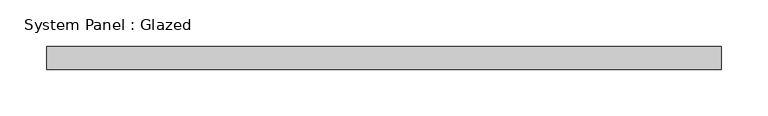
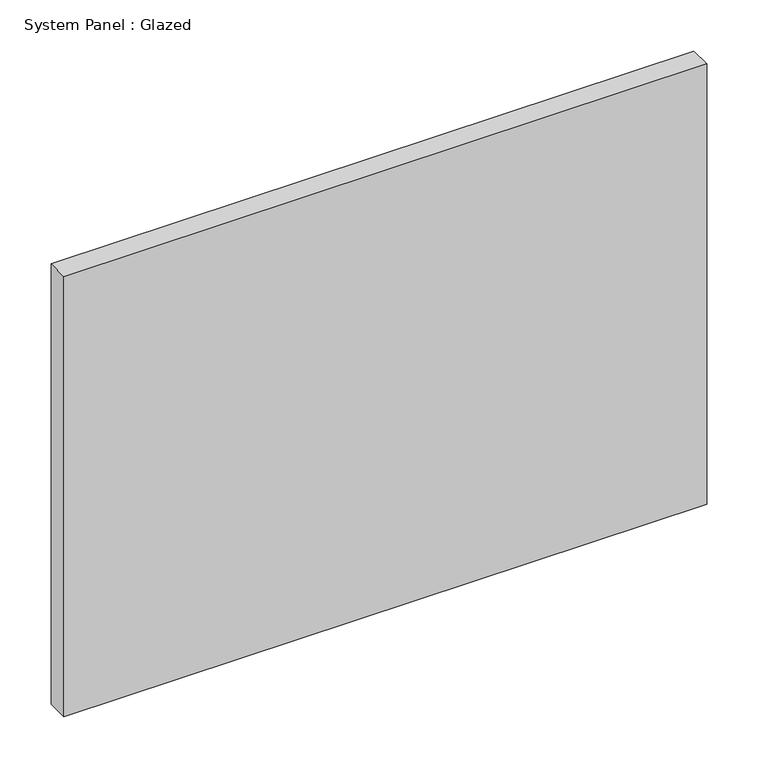
"""IFC4 building model written with IfcOpenShell, lengths in millimetres: plate geometry, System Panel : Glazed."""

from ifc_helpers import new_model, si_unit, origin, origin_with_axes, place, context, project, spatial, polyline, outline, extrude, source, transform, mapped, element, save


def system_panel_glazed_f19c5426(model_context):
    return source(origin(), model_context, "Body", "SweptSolid", [
        extrude(outline(polyline([(362.5, 24.5), (-362.5, 24.5), (-362.5, 49.5), (362.5, 49.5), (362.5, 24.5)])), origin_with_axes(), (0.0, 0.0, 1.0), 525.0),
    ])


if __name__ == "__main__":
    model = new_model("IFC4")
    model_context = context("Model", 3, world=origin())
    ifc_project = project(units=[si_unit("LENGTHUNIT", "METRE", prefix="MILLI")], contexts=[model_context])
    site = spatial("IfcSite", under=ifc_project)
    building = spatial("IfcBuilding", under=site)
    placement = place(None, origin())
    system_panel_glazed_shape = system_panel_glazed_f19c5426(model_context)
    element("IfcPlate", 1, ObjectType="System Panel : Glazed", at=placement, inside=building, context=model_context, shape_type="MappedRepresentation", body=[
        mapped(system_panel_glazed_shape, transform((0.0, 0.0, 0.0), x_axis=(1.0, 0.0, 0.0), y_axis=(0.0, 1.0, 0.0), z_axis=(0.0, 0.0, 1.0))),
    ])
    save(model, "model.ifc")

# Revit data of these elements
# Type "System Panel : Glazed"
#   Construction Type Id = "GSP4R"
#   Analytic Construction = "1/8 in Pilkington single glazing"
#   Visual Light Transmittance = 0.9
#   Solar Heat Gain Coefficient = 0.86
#   Heat Transfer Coefficient (U) = 6.7069 W/(m²·K)
#   Define Thermal Properties by = 1
# Element 1 (IfcPlate, "System Panel : Glazed")
#   Materials on its faces: "Glass"
# Materials
#   "Glass": class "Glass", colour RGB 245 245 243, transparency 1, Description = "Soda Lime Glass", Cost = 0
